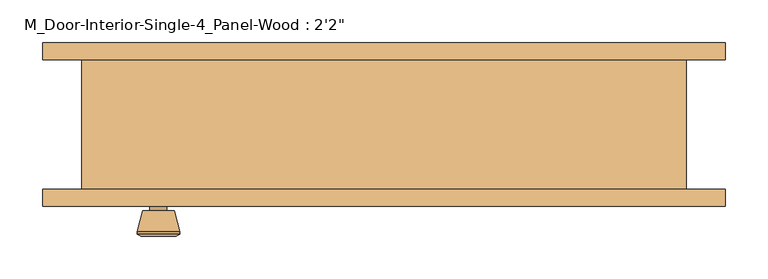
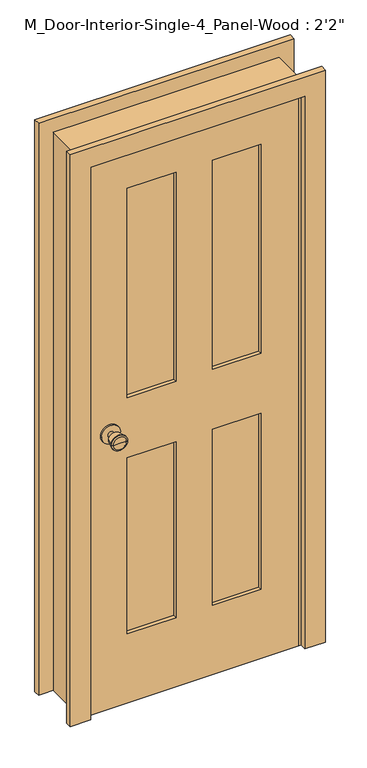
"""IFC4 building model written with IfcOpenShell, lengths in millimetres: door geometry."""

from ifc_helpers import new_model, si_unit, point, frame, frame_2d, origin, place, context, project, spatial, polyline, circle_curve, trimmed, segment, composite_curve, outline, extrude, faceted_brep, source, transform, mapped, element, save
from ifc_brep_helpers import plane_surface, cylinder_surface, revolved_surface, advanced_brep


def door_7109d6db(model_context):
    return source(origin(), model_context, "Body", "SolidModel", [
        advanced_brep(
        [(-265.2, -32.025, 914.4), (-275.2, -32.025, 914.4), (-255.2, -32.025, 914.4), (-244.7241324, 16.975, 914.4), (-285.6758676, 16.975, 914.4), (-265.2, 16.975, 914.4), (-240.2, 15.1471319, 914.4), (-290.2, 15.1471319, 914.4), (-240.2, 11.6834537, 914.4), (-290.2, 11.6834537, 914.4), (-246.563764, -13.025, 914.4), (-283.836236, -13.025, 914.4), (-255.2, -13.025, 914.4), (-275.2, -13.025, 914.4)],
        [
            (0, 1),
            (1, 2, circle_curve(frame((-265.2, -32.025, 914.4), z_axis=(0.0, -1.0, 0.0), x_axis=(-1.0, 0.0, 0.0)), 10.0)),
            (2, 0),
            (2, 1, circle_curve(frame((-265.2, -32.025, 914.4), z_axis=(0.0, -1.0, 0.0), x_axis=(-1.0, 0.0, 0.0)), 10.0)),
            (3, 4, circle_curve(frame((-265.2, 16.975, 914.4), z_axis=(0.0, 1.0, 0.0), x_axis=(-1.0, 0.0, 0.0)), 20.4758676)),
            (4, 5),
            (5, 3),
            (4, 3, circle_curve(frame((-265.2, 16.975, 914.4), z_axis=(0.0, 1.0, 0.0), x_axis=(-1.0, 0.0, 0.0)), 20.4758676)),
            (6, 7, circle_curve(frame((-265.2, 15.1471319, 914.4), z_axis=(0.0, 1.0, 0.0), x_axis=(-1.0, 0.0, 0.0)), 25.0)),
            (7, 4),
            (3, 6),
            (7, 6, circle_curve(frame((-265.2, 15.1471319, 914.4), z_axis=(0.0, 1.0, 0.0), x_axis=(-1.0, 0.0, 0.0)), 25.0)),
            (8, 9, circle_curve(frame((-265.2, 11.6834537, 914.4), z_axis=(0.0, 1.0, 0.0), x_axis=(-1.0, 0.0, 0.0)), 25.0)),
            (9, 7),
            (6, 8),
            (9, 8, circle_curve(frame((-265.2, 11.6834537, 914.4), z_axis=(0.0, 1.0, 0.0), x_axis=(-1.0, 0.0, 0.0)), 25.0)),
            (10, 11, circle_curve(frame((-265.2, -13.025, 914.4), z_axis=(0.0, 1.0, 0.0), x_axis=(-1.0, 0.0, 0.0)), 18.636236)),
            (11, 9),
            (8, 10),
            (11, 10, circle_curve(frame((-265.2, -13.025, 914.4), z_axis=(0.0, 1.0, 0.0), x_axis=(-1.0, 0.0, 0.0)), 18.636236)),
            (12, 13, circle_curve(frame((-265.2, -13.025, 914.4), z_axis=(0.0, 1.0, 0.0), x_axis=(-1.0, 0.0, 0.0)), 10.0)),
            (13, 11),
            (10, 12),
            (13, 12, circle_curve(frame((-265.2, -13.025, 914.4), z_axis=(0.0, 1.0, 0.0), x_axis=(-1.0, 0.0, 0.0)), 10.0)),
            (1, 13),
            (12, 2),
        ],
        [
            plane_surface(frame((-265.2, -32.025, 914.4), z_axis=(0.0, -1.0, 0.0), x_axis=(-1.0, 0.0, 0.0))),
            plane_surface(frame((-265.2, 16.975, 914.4), z_axis=(0.0, 1.0, 0.0), x_axis=(-1.0, 0.0, 0.0))),
            revolved_surface(polyline([(-285.6758676, 16.975, 914.4), (-290.2, 15.1471319, 914.4)]), (-265.2, -32.025, 914.4), (0.0, -1.0, 0.0)),
            cylinder_surface(frame((-265.2, -32.025, 914.4), z_axis=(0.0, -1.0, 0.0), x_axis=(-1.0, 0.0, 0.0)), 25.0),
            revolved_surface(polyline([(-290.2, 11.6834537, 914.4), (-283.836236, -13.025, 914.4)]), (-265.2, -32.025, 914.4), (0.0, -1.0, 0.0)),
            plane_surface(frame((-265.2, -13.025, 914.4), z_axis=(0.0, -1.0, 0.0), x_axis=(-1.0, 0.0, 0.0))),
            cylinder_surface(frame((-265.2, -32.025, 914.4), z_axis=(0.0, -1.0, 0.0), x_axis=(-1.0, 0.0, 0.0)), 10.0),
        ],
        [
            (0, [[1, 2, 3]]),
            (0, [[-3, 4, -1]]),
            (1, [[5, 6, 7]]),
            (1, [[8, -7, -6]]),
            (2, [[9, 10, -5, 11]]),
            (2, [[12, -11, -8, -10]]),
            (3, [[13, 14, -9, 15]]),
            (3, [[16, -15, -12, -14]]),
            (4, [[17, 18, -13, 19]]),
            (4, [[20, -19, -16, -18]]),
            (5, [[21, 22, -17, 23]]),
            (5, [[24, -23, -20, -22]]),
            (6, [[-2, 25, -21, 26]]),
            (6, [[-4, -26, -24, -25]]),
        ],
    ),
        extrude(outline(composite_curve([segment(trimmed(circle_curve(frame_2d((914.4, -265.2)), 30.0), [point((914.4, -295.2))], [point((914.4, -235.2))], False, "CARTESIAN"), True, "CONTINUOUS"), segment(trimmed(circle_curve(frame_2d((914.4, -265.2)), 30.0), [point((914.4, -235.2))], [point((914.4, -295.2))], False, "CARTESIAN"), True, "CONTINUOUS")], self_intersect=False)), frame((0.0, -38.025, 0.0), z_axis=(0.0, 1.0, 0.0), x_axis=(0.0, 0.0, 1.0)), (0.0, 0.0, 1.0), 6.0),
        advanced_brep(
        [(-265.2, -79.025, 914.4), (-255.2, -79.025, 914.4), (-275.2, -79.025, 914.4), (-244.7241324, -128.025, 914.4), (-265.2, -128.025, 914.4), (-285.6758676, -128.025, 914.4), (-240.2, -126.1971319, 914.4), (-290.2, -126.1971319, 914.4), (-240.2, -122.7334537, 914.4), (-290.2, -122.7334537, 914.4), (-246.563764, -98.025, 914.4), (-283.836236, -98.025, 914.4), (-255.2, -98.025, 914.4), (-275.2, -98.025, 914.4)],
        [
            (0, 1),
            (1, 2, circle_curve(frame((-265.2, -79.025, 914.4), z_axis=(0.0, 1.0, 0.0), x_axis=(-1.0, 0.0, 0.0)), 10.0)),
            (2, 0),
            (2, 1, circle_curve(frame((-265.2, -79.025, 914.4), z_axis=(0.0, 1.0, 0.0), x_axis=(-1.0, 0.0, 0.0)), 10.0)),
            (3, 4),
            (4, 5),
            (5, 3, circle_curve(frame((-265.2, -128.025, 914.4), z_axis=(0.0, -1.0, 0.0), x_axis=(-1.0, 0.0, 0.0)), 20.4758676)),
            (3, 5, circle_curve(frame((-265.2, -128.025, 914.4), z_axis=(0.0, -1.0, 0.0), x_axis=(-1.0, 0.0, 0.0)), 20.4758676)),
            (6, 3),
            (5, 7),
            (7, 6, circle_curve(frame((-265.2, -126.1971319, 914.4), z_axis=(0.0, -1.0, 0.0), x_axis=(-1.0, 0.0, 0.0)), 25.0)),
            (6, 7, circle_curve(frame((-265.2, -126.1971319, 914.4), z_axis=(0.0, -1.0, 0.0), x_axis=(-1.0, 0.0, 0.0)), 25.0)),
            (8, 6),
            (7, 9),
            (9, 8, circle_curve(frame((-265.2, -122.7334537, 914.4), z_axis=(0.0, -1.0, 0.0), x_axis=(-1.0, 0.0, 0.0)), 25.0)),
            (8, 9, circle_curve(frame((-265.2, -122.7334537, 914.4), z_axis=(0.0, -1.0, 0.0), x_axis=(-1.0, 0.0, 0.0)), 25.0)),
            (10, 8),
            (9, 11),
            (11, 10, circle_curve(frame((-265.2, -98.025, 914.4), z_axis=(0.0, -1.0, 0.0), x_axis=(-1.0, 0.0, 0.0)), 18.636236)),
            (10, 11, circle_curve(frame((-265.2, -98.025, 914.4), z_axis=(0.0, -1.0, 0.0), x_axis=(-1.0, 0.0, 0.0)), 18.636236)),
            (12, 10),
            (11, 13),
            (13, 12, circle_curve(frame((-265.2, -98.025, 914.4), z_axis=(0.0, -1.0, 0.0), x_axis=(-1.0, 0.0, 0.0)), 10.0)),
            (12, 13, circle_curve(frame((-265.2, -98.025, 914.4), z_axis=(0.0, -1.0, 0.0), x_axis=(-1.0, 0.0, 0.0)), 10.0)),
            (1, 12),
            (13, 2),
        ],
        [
            plane_surface(frame((-265.2, -79.025, 914.4), z_axis=(0.0, 1.0, 0.0), x_axis=(-1.0, 0.0, 0.0))),
            plane_surface(frame((-265.2, -128.025, 914.4), z_axis=(0.0, -1.0, 0.0), x_axis=(-1.0, 0.0, 0.0))),
            revolved_surface(polyline([(-285.6758676, -128.025, 914.4), (-290.2, -126.1971319, 914.4)]), (-265.2, -79.025, 914.4), (0.0, 1.0, 0.0)),
            cylinder_surface(frame((-265.2, -79.025, 914.4), z_axis=(0.0, 1.0, 0.0), x_axis=(-1.0, 0.0, 0.0)), 25.0),
            revolved_surface(polyline([(-290.2, -122.7334537, 914.4), (-283.836236, -98.025, 914.4)]), (-265.2, -79.025, 914.4), (0.0, 1.0, 0.0)),
            plane_surface(frame((-265.2, -98.025, 914.4), z_axis=(0.0, 1.0, 0.0), x_axis=(-1.0, 0.0, 0.0))),
            cylinder_surface(frame((-265.2, -79.025, 914.4), z_axis=(0.0, 1.0, 0.0), x_axis=(-1.0, 0.0, 0.0)), 10.0),
        ],
        [
            (0, [[1, 2, 3]]),
            (0, [[-3, 4, -1]]),
            (1, [[5, 6, 7]]),
            (1, [[-6, -5, 8]]),
            (2, [[9, -7, 10, 11]]),
            (2, [[-10, -8, -9, 12]]),
            (3, [[13, -11, 14, 15]]),
            (3, [[-14, -12, -13, 16]]),
            (4, [[17, -15, 18, 19]]),
            (4, [[-18, -16, -17, 20]]),
            (5, [[21, -19, 22, 23]]),
            (5, [[-22, -20, -21, 24]]),
            (6, [[25, -23, 26, -2]]),
            (6, [[-26, -24, -25, -4]]),
        ],
    ),
        extrude(outline(composite_curve([segment(trimmed(circle_curve(frame_2d((914.4, -265.2)), 30.0), [point((914.4, -295.2))], [point((914.4, -235.2))], False, "CARTESIAN"), True, "CONTINUOUS"), segment(trimmed(circle_curve(frame_2d((914.4, -265.2)), 30.0), [point((914.4, -235.2))], [point((914.4, -295.2))], False, "CARTESIAN"), True, "CONTINUOUS")], self_intersect=False)), frame((0.0, -79.025, 0.0), z_axis=(0.0, 1.0, 0.0), x_axis=(0.0, 0.0, 1.0)), (0.0, 0.0, 1.0), 6.0),
        faceted_brep([(355.2, -73.025, 0.0), (330.2, -73.025, 0.0), (330.2, -38.025, 0.0), (317.5, -38.025, 0.0), (317.5, -3.1, 0.0), (330.2, -3.1, 0.0), (330.2, 79.375, 0.0), (355.2, 79.375, 0.0), (355.2, 79.375, 1853.8), (355.2, -73.025, 1853.8), (330.2, 79.375, 1828.8), (-330.2, 79.375, 1828.8), (-330.2, 79.375, 0.0), (-355.2, 79.375, 0.0), (-355.2, 79.375, 1853.8), (330.2, -3.1, 1828.8), (317.5, -3.1, 1816.1), (-317.5, -3.1, 1816.1), (-317.5, -3.1, 0.0), (-330.2, -3.1, 0.0), (-330.2, -3.1, 1828.8), (317.5, -38.025, 1816.1), (330.2, -38.025, 1828.8), (-330.2, -38.025, 1828.8), (-330.2, -38.025, 0.0), (-317.5, -38.025, 0.0), (-317.5, -38.025, 1816.1), (330.2, -73.025, 1828.8), (-355.2, -73.025, 1853.8), (-355.2, -73.025, 0.0), (-330.2, -73.025, 0.0), (-330.2, -73.025, 1828.8)], [[[0, 1, 2, 3, 4, 5, 6, 7]], [[7, 8, 9, 0]], [[6, 10, 11, 12, 13, 14, 8, 7]], [[5, 15, 10, 6]], [[4, 16, 17, 18, 19, 20, 15, 5]], [[3, 21, 16, 4]], [[2, 22, 23, 24, 25, 26, 21, 3]], [[1, 27, 22, 2]], [[0, 9, 28, 29, 30, 31, 27, 1]], [[8, 14, 28, 9]], [[15, 20, 11, 10]], [[21, 26, 17, 16]], [[27, 31, 23, 22]], [[29, 13, 12, 19, 18, 25, 24, 30]], [[14, 13, 29, 28]], [[20, 19, 12, 11]], [[26, 25, 18, 17]], [[31, 30, 24, 23]]]),
        extrude(outline(polyline([(1828.8, -330.2), (0.0, -330.2), (0.0, 330.2), (1828.8, 330.2), (1828.8, -330.2)]), holes=[polyline([(1708.8, 57.5), (1708.8, 210.2), (1014.4, 210.2), (1014.4, 57.5), (1708.8, 57.5)]), polyline([(1014.4, -57.5), (1014.4, -210.2), (1708.8, -210.2), (1708.8, -57.5), (1014.4, -57.5)]), polyline([(814.4, 57.5), (814.4, 210.2), (230.0, 210.2), (230.0, 57.5), (814.4, 57.5)]), polyline([(230.0, -57.5), (230.0, -210.2), (814.4, -210.2), (814.4, -57.5), (230.0, -57.5)])]), frame((0.0, -73.025, 0.0), z_axis=(0.0, 1.0, 0.0), x_axis=(0.0, 0.0, 1.0)), (0.0, 0.0, 1.0), 35.0),
        extrude(outline(polyline([(210.2, -49.6916667), (210.2, -61.3583333), (57.5, -61.3583333), (57.5, -49.6916667), (210.2, -49.6916667)])), frame((0.0, 0.0, 1014.4), z_axis=(0.0, 0.0, 1.0), x_axis=(1.0, 0.0, 0.0)), (0.0, 0.0, 1.0), 694.4),
        extrude(outline(polyline([(-57.5, -49.6916667), (-57.5, -61.3583333), (-210.2, -61.3583333), (-210.2, -49.6916667), (-57.5, -49.6916667)])), frame((0.0, 0.0, 1014.4), z_axis=(0.0, 0.0, 1.0), x_axis=(1.0, 0.0, 0.0)), (0.0, 0.0, 1.0), 694.4),
        extrude(outline(polyline([(210.2, -49.6916667), (210.2, -61.3583333), (57.5, -61.3583333), (57.5, -49.6916667), (210.2, -49.6916667)])), frame((0.0, 0.0, 230.0), z_axis=(0.0, 0.0, 1.0), x_axis=(1.0, 0.0, 0.0)), (0.0, 0.0, 1.0), 584.4),
        extrude(outline(polyline([(-57.5, -49.6916667), (-57.5, -61.3583333), (-210.2, -61.3583333), (-210.2, -49.6916667), (-57.5, -49.6916667)])), frame((0.0, 0.0, 230.0), z_axis=(0.0, 0.0, 1.0), x_axis=(1.0, 0.0, 0.0)), (0.0, 0.0, 1.0), 584.4),
        extrude(outline(polyline([(0.0, 401.55), (1900.15, 401.55), (1900.15, -401.55), (0.0, -401.55), (0.0, -336.55), (1835.15, -336.55), (1835.15, 336.55), (0.0, 336.55), (0.0, 401.55)])), frame((0.0, -93.025, 0.0), z_axis=(0.0, 1.0, 0.0), x_axis=(0.0, 0.0, 1.0)), (0.0, 0.0, 1.0), 20.0),
        extrude(outline(polyline([(0.0, 401.55), (1900.15, 401.55), (1900.15, -401.55), (0.0, -401.55), (0.0, -336.55), (1835.15, -336.55), (1835.15, 336.55), (0.0, 336.55), (0.0, 401.55)])), frame((0.0, 79.375, 0.0), z_axis=(0.0, 1.0, 0.0), x_axis=(0.0, 0.0, 1.0)), (0.0, 0.0, 1.0), 20.0),
    ])


if __name__ == "__main__":
    model = new_model("IFC4")
    model_context = context("Model", 3, world=origin())
    ifc_project = project(units=[si_unit("LENGTHUNIT", "METRE", prefix="MILLI")], contexts=[model_context])
    site = spatial("IfcSite", under=ifc_project)
    building = spatial("IfcBuilding", under=site)
    placement = place(None, origin())
    door_shape = door_7109d6db(model_context)
    element("IfcDoor", 1, ObjectType="M_Door-Interior-Single-4_Panel-Wood : 2'2\"", at=placement, inside=building, context=model_context, shape_type="MappedRepresentation", body=[
        mapped(door_shape, transform((0.0, 0.0, 0.0), x_axis=(1.0, 0.0, 0.0), y_axis=(0.0, 1.0, 0.0), z_axis=(0.0, 0.0, 1.0))),
    ])
    save(model, "model.ifc")

# Revit data of these elements
# Type "M_Door-Interior-Single-4_Panel-Wood : 2'2\""
#   Type Mark = "43"
#   Assembly Code = "C1020300"
#   Analytic Construction = "Wooden"
#   Top Rail = 0' - 4.72441"
#   Thickness = 0' - 1.37795"
#   Thermal Resistance (R) = 0.455703 (m²·K)/W
#   Swing Angle [instance default] = 90.00°
#   Stiles = 0' - 4.72441"
#   Rough Width = 2' - 3.9685"
#   Rough Height = 6' - 0.98425"
#   Mullion = 0' - 4.52756"
#   Lock Rail = 0' - 7.87402"
#   Height = 6' - 0"
#   Width = 2' - 2"
#   Heat Transfer Coefficient (U) = 2.19465 W/(m²·K)
#   Bottom Rail = 0' - 9.05512"
#   Trim Material = Cherry
#   Panel Material = Cherry
#   Frame Material = Cherry
#   Door Handle Material = Aluminum
#   Visual Light Transmittance = 0
#   Solar Heat Gain Coefficient = 0
#   Wall Closure = (empty or 0)
#   Function = (empty or 0)
# Element 1 (IfcDoor, "M_Door-Interior-Single-4_Panel-Wood : 2'2\"")
#   Materials on its faces: "Cherry", "Aluminum"
# Materials
#   "Cherry": class "Wood", colour RGB 226 177 128, transparency 0, Description = "Prunus Serotina", Cost = 0
#   "Aluminum": class "Metal", colour RGB 247 247 247, transparency 0, Description = "Aluminum 6061", Cost = 0
